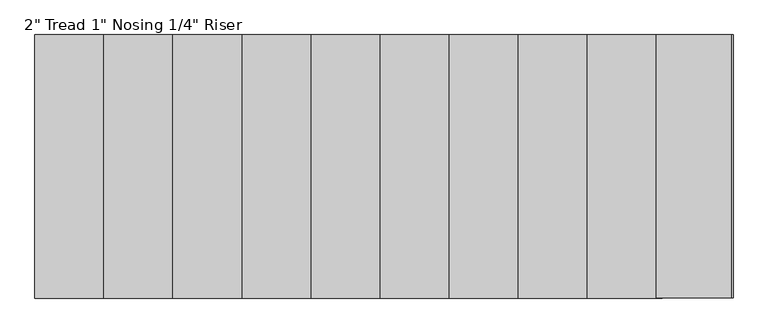
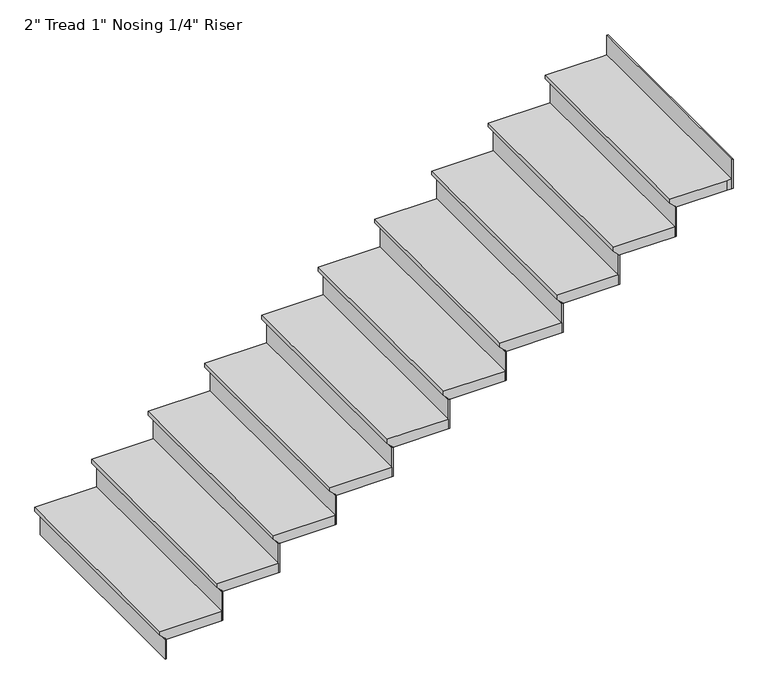
"""IFC4 building model written with IfcOpenShell, lengths in millimetres: stair flight geometry."""

from ifc_helpers import new_model, si_unit, origin, place, context, project, spatial, faceted_brep, source, transform, mapped, element, save


def stair_flight_cc90426c(model_context):
    return source(origin(), model_context, "Body", "Brep", [
        faceted_brep([(-459.26646, -1849.1834702, 133.35), (-459.26646, -1849.1834702, 152.4), (-459.26646, -782.3834702, 152.4), (-459.26646, -782.3834702, 133.35), (-433.86646, -1849.1834702, 107.95), (-433.86646, -782.3834702, 107.95), (-154.46646, -1849.1834702, 152.4), (-154.46646, -782.3834702, 152.4), (-433.86646, -782.3834702, 101.6), (-154.46646, -782.3834702, 101.6), (-154.46646, -1849.1834702, 101.6), (-433.86646, -1849.1834702, 101.6)], [[[0, 1, 2, 3]], [[4, 0, 3, 5]], [[2, 1, 6, 7]], [[8, 9, 10, 11]], [[2, 7, 9, 8, 5, 3]], [[8, 11, 4, 5]], [[6, 1, 0, 4, 11, 10]], [[7, 6, 10, 9]]]),
        faceted_brep([(-433.86646, -1849.1834702, 101.6), (-433.86646, -1849.1834702, 0.0), (-427.51646, -1849.1834702, 0.0), (-427.51646, -1849.1834702, 101.6), (-433.86646, -782.3834702, 101.6), (-427.51646, -782.3834702, 101.6), (-427.51646, -782.3834702, 0.0), (-433.86646, -782.3834702, 0.0)], [[[0, 1, 2, 3]], [[4, 5, 6, 7]], [[1, 0, 4, 7]], [[2, 1, 7, 6]], [[3, 2, 6, 5]], [[0, 3, 5, 4]]]),
        faceted_brep([(-154.46646, -1849.1834702, 254.0), (-154.46646, -1849.1834702, 101.6), (-148.11646, -1849.1834702, 101.6), (-148.11646, -1849.1834702, 254.0), (-154.46646, -782.3834702, 254.0), (-148.11646, -782.3834702, 254.0), (-148.11646, -782.3834702, 101.6), (-154.46646, -782.3834702, 101.6)], [[[0, 1, 2, 3]], [[4, 5, 6, 7]], [[1, 0, 4, 7]], [[2, 1, 7, 6]], [[3, 2, 6, 5]], [[0, 3, 5, 4]]]),
        faceted_brep([(-179.86646, -782.3834702, 304.8), (-179.86646, -1849.1834702, 304.8), (124.93354, -1849.1834702, 304.8), (124.93354, -782.3834702, 304.8), (-154.46646, -782.3834702, 254.0), (124.93354, -782.3834702, 254.0), (124.93354, -1849.1834702, 254.0), (-154.46646, -1849.1834702, 254.0), (-154.46646, -782.3834702, 260.35), (-179.86646, -782.3834702, 285.75), (-154.46646, -1849.1834702, 260.35), (-179.86646, -1849.1834702, 285.75)], [[[0, 1, 2, 3]], [[4, 5, 6, 7]], [[0, 3, 5, 4, 8, 9]], [[4, 7, 10, 8]], [[2, 1, 11, 10, 7, 6]], [[3, 2, 6, 5]], [[11, 1, 0, 9]], [[10, 11, 9, 8]]]),
        faceted_brep([(124.93354, -1849.1834702, 406.4), (124.93354, -1849.1834702, 254.0), (131.28354, -1849.1834702, 254.0), (131.28354, -1849.1834702, 406.4), (124.93354, -782.3834702, 406.4), (131.28354, -782.3834702, 406.4), (131.28354, -782.3834702, 254.0), (124.93354, -782.3834702, 254.0)], [[[0, 1, 2, 3]], [[4, 5, 6, 7]], [[1, 0, 4, 7]], [[2, 1, 7, 6]], [[3, 2, 6, 5]], [[0, 3, 5, 4]]]),
        faceted_brep([(99.53354, -782.3834702, 457.2), (99.53354, -1849.1834702, 457.2), (404.33354, -1849.1834702, 457.2), (404.33354, -782.3834702, 457.2), (124.93354, -782.3834702, 406.4), (404.33354, -782.3834702, 406.4), (404.33354, -1849.1834702, 406.4), (124.93354, -1849.1834702, 406.4), (124.93354, -782.3834702, 412.75), (99.53354, -782.3834702, 438.15), (124.93354, -1849.1834702, 412.75), (99.53354, -1849.1834702, 438.15)], [[[0, 1, 2, 3]], [[4, 5, 6, 7]], [[0, 3, 5, 4, 8, 9]], [[4, 7, 10, 8]], [[2, 1, 11, 10, 7, 6]], [[3, 2, 6, 5]], [[11, 1, 0, 9]], [[10, 11, 9, 8]]]),
        faceted_brep([(404.33354, -1849.1834702, 558.8), (404.33354, -1849.1834702, 406.4), (410.68354, -1849.1834702, 406.4), (410.68354, -1849.1834702, 558.8), (404.33354, -782.3834702, 558.8), (410.68354, -782.3834702, 558.8), (410.68354, -782.3834702, 406.4), (404.33354, -782.3834702, 406.4)], [[[0, 1, 2, 3]], [[4, 5, 6, 7]], [[1, 0, 4, 7]], [[2, 1, 7, 6]], [[3, 2, 6, 5]], [[0, 3, 5, 4]]]),
        faceted_brep([(378.93354, -782.3834702, 609.6), (378.93354, -1849.1834702, 609.6), (683.73354, -1849.1834702, 609.6), (683.73354, -782.3834702, 609.6), (404.33354, -782.3834702, 558.8), (683.73354, -782.3834702, 558.8), (683.73354, -1849.1834702, 558.8), (404.33354, -1849.1834702, 558.8), (404.33354, -782.3834702, 565.15), (378.93354, -782.3834702, 590.55), (404.33354, -1849.1834702, 565.15), (378.93354, -1849.1834702, 590.55)], [[[0, 1, 2, 3]], [[4, 5, 6, 7]], [[0, 3, 5, 4, 8, 9]], [[4, 7, 10, 8]], [[2, 1, 11, 10, 7, 6]], [[3, 2, 6, 5]], [[11, 1, 0, 9]], [[10, 11, 9, 8]]]),
        faceted_brep([(683.73354, -1849.1834702, 711.2), (683.73354, -1849.1834702, 558.8), (690.08354, -1849.1834702, 558.8), (690.08354, -1849.1834702, 711.2), (683.73354, -782.3834702, 711.2), (690.08354, -782.3834702, 711.2), (690.08354, -782.3834702, 558.8), (683.73354, -782.3834702, 558.8)], [[[0, 1, 2, 3]], [[4, 5, 6, 7]], [[1, 0, 4, 7]], [[2, 1, 7, 6]], [[3, 2, 6, 5]], [[0, 3, 5, 4]]]),
        faceted_brep([(658.33354, -782.3834702, 762.0), (658.33354, -1849.1834702, 762.0), (963.13354, -1849.1834702, 762.0), (963.13354, -782.3834702, 762.0), (683.73354, -782.3834702, 711.2), (963.13354, -782.3834702, 711.2), (963.13354, -1849.1834702, 711.2), (683.73354, -1849.1834702, 711.2), (683.73354, -782.3834702, 717.55), (658.33354, -782.3834702, 742.95), (683.73354, -1849.1834702, 717.55), (658.33354, -1849.1834702, 742.95)], [[[0, 1, 2, 3]], [[4, 5, 6, 7]], [[0, 3, 5, 4, 8, 9]], [[4, 7, 10, 8]], [[2, 1, 11, 10, 7, 6]], [[3, 2, 6, 5]], [[11, 1, 0, 9]], [[10, 11, 9, 8]]]),
        faceted_brep([(963.13354, -1849.1834702, 863.6), (963.13354, -1849.1834702, 711.2), (969.48354, -1849.1834702, 711.2), (969.48354, -1849.1834702, 863.6), (963.13354, -782.3834702, 863.6), (969.48354, -782.3834702, 863.6), (969.48354, -782.3834702, 711.2), (963.13354, -782.3834702, 711.2)], [[[0, 1, 2, 3]], [[4, 5, 6, 7]], [[1, 0, 4, 7]], [[2, 1, 7, 6]], [[3, 2, 6, 5]], [[0, 3, 5, 4]]]),
        faceted_brep([(937.73354, -782.3834702, 914.4), (937.73354, -1849.1834702, 914.4), (1242.53354, -1849.1834702, 914.4), (1242.53354, -782.3834702, 914.4), (963.13354, -782.3834702, 863.6), (1242.53354, -782.3834702, 863.6), (1242.53354, -1849.1834702, 863.6), (963.13354, -1849.1834702, 863.6), (963.13354, -782.3834702, 869.95), (937.73354, -782.3834702, 895.35), (963.13354, -1849.1834702, 869.95), (937.73354, -1849.1834702, 895.35)], [[[0, 1, 2, 3]], [[4, 5, 6, 7]], [[0, 3, 5, 4, 8, 9]], [[4, 7, 10, 8]], [[2, 1, 11, 10, 7, 6]], [[3, 2, 6, 5]], [[11, 1, 0, 9]], [[10, 11, 9, 8]]]),
        faceted_brep([(1242.53354, -1849.1834702, 1016.0), (1242.53354, -1849.1834702, 863.6), (1248.88354, -1849.1834702, 863.6), (1248.88354, -1849.1834702, 1016.0), (1242.53354, -782.3834702, 1016.0), (1248.88354, -782.3834702, 1016.0), (1248.88354, -782.3834702, 863.6), (1242.53354, -782.3834702, 863.6)], [[[0, 1, 2, 3]], [[4, 5, 6, 7]], [[1, 0, 4, 7]], [[2, 1, 7, 6]], [[3, 2, 6, 5]], [[0, 3, 5, 4]]]),
        faceted_brep([(1217.13354, -782.3834702, 1066.8), (1217.13354, -1849.1834702, 1066.8), (1521.93354, -1849.1834702, 1066.8), (1521.93354, -782.3834702, 1066.8), (1242.53354, -782.3834702, 1016.0), (1521.93354, -782.3834702, 1016.0), (1521.93354, -1849.1834702, 1016.0), (1242.53354, -1849.1834702, 1016.0), (1242.53354, -782.3834702, 1022.35), (1217.13354, -782.3834702, 1047.75), (1242.53354, -1849.1834702, 1022.35), (1217.13354, -1849.1834702, 1047.75)], [[[0, 1, 2, 3]], [[4, 5, 6, 7]], [[0, 3, 5, 4, 8, 9]], [[4, 7, 10, 8]], [[2, 1, 11, 10, 7, 6]], [[3, 2, 6, 5]], [[11, 1, 0, 9]], [[10, 11, 9, 8]]]),
        faceted_brep([(1521.93354, -1849.1834702, 1168.4), (1521.93354, -1849.1834702, 1016.0), (1528.28354, -1849.1834702, 1016.0), (1528.28354, -1849.1834702, 1168.4), (1521.93354, -782.3834702, 1168.4), (1528.28354, -782.3834702, 1168.4), (1528.28354, -782.3834702, 1016.0), (1521.93354, -782.3834702, 1016.0)], [[[0, 1, 2, 3]], [[4, 5, 6, 7]], [[1, 0, 4, 7]], [[2, 1, 7, 6]], [[3, 2, 6, 5]], [[0, 3, 5, 4]]]),
        faceted_brep([(1496.53354, -782.3834702, 1219.2), (1496.53354, -1849.1834702, 1219.2), (1801.33354, -1849.1834702, 1219.2), (1801.33354, -782.3834702, 1219.2), (1521.93354, -782.3834702, 1168.4), (1801.33354, -782.3834702, 1168.4), (1801.33354, -1849.1834702, 1168.4), (1521.93354, -1849.1834702, 1168.4), (1521.93354, -782.3834702, 1174.75), (1496.53354, -782.3834702, 1200.15), (1521.93354, -1849.1834702, 1174.75), (1496.53354, -1849.1834702, 1200.15)], [[[0, 1, 2, 3]], [[4, 5, 6, 7]], [[0, 3, 5, 4, 8, 9]], [[4, 7, 10, 8]], [[2, 1, 11, 10, 7, 6]], [[3, 2, 6, 5]], [[11, 1, 0, 9]], [[10, 11, 9, 8]]]),
        faceted_brep([(1801.33354, -1849.1834702, 1320.8), (1801.33354, -1849.1834702, 1168.4), (1807.68354, -1849.1834702, 1168.4), (1807.68354, -1849.1834702, 1320.8), (1801.33354, -782.3834702, 1320.8), (1807.68354, -782.3834702, 1320.8), (1807.68354, -782.3834702, 1168.4), (1801.33354, -782.3834702, 1168.4)], [[[0, 1, 2, 3]], [[4, 5, 6, 7]], [[1, 0, 4, 7]], [[2, 1, 7, 6]], [[3, 2, 6, 5]], [[0, 3, 5, 4]]]),
        faceted_brep([(1775.93354, -782.3834702, 1371.6), (1775.93354, -1849.1834702, 1371.6), (2080.73354, -1849.1834702, 1371.6), (2080.73354, -782.3834702, 1371.6), (1801.33354, -782.3834702, 1320.8), (2080.73354, -782.3834702, 1320.8), (2080.73354, -1849.1834702, 1320.8), (1801.33354, -1849.1834702, 1320.8), (1801.33354, -782.3834702, 1327.15), (1775.93354, -782.3834702, 1352.55), (1801.33354, -1849.1834702, 1327.15), (1775.93354, -1849.1834702, 1352.55)], [[[0, 1, 2, 3]], [[4, 5, 6, 7]], [[0, 3, 5, 4, 8, 9]], [[4, 7, 10, 8]], [[2, 1, 11, 10, 7, 6]], [[3, 2, 6, 5]], [[11, 1, 0, 9]], [[10, 11, 9, 8]]]),
        faceted_brep([(2360.13354, -1849.1834702, 1625.6), (2360.13354, -1849.1834702, 1473.2), (2366.48354, -1849.1834702, 1473.2), (2366.48354, -1849.1834702, 1625.6), (2360.13354, -782.3834702, 1625.6), (2366.48354, -782.3834702, 1625.6), (2366.48354, -782.3834702, 1473.2), (2360.13354, -782.3834702, 1473.2)], [[[0, 1, 2, 3]], [[4, 5, 6, 7]], [[1, 0, 4, 7]], [[2, 1, 7, 6]], [[3, 2, 6, 5]], [[0, 3, 5, 4]]]),
        faceted_brep([(2080.73354, -1849.1834702, 1473.2), (2080.73354, -1849.1834702, 1320.8), (2087.08354, -1849.1834702, 1320.8), (2087.08354, -1849.1834702, 1473.2), (2080.73354, -782.3834702, 1473.2), (2087.08354, -782.3834702, 1473.2), (2087.08354, -782.3834702, 1320.8), (2080.73354, -782.3834702, 1320.8)], [[[0, 1, 2, 3]], [[4, 5, 6, 7]], [[1, 0, 4, 7]], [[2, 1, 7, 6]], [[3, 2, 6, 5]], [[0, 3, 5, 4]]]),
        faceted_brep([(2360.13354, -782.3834702, 1524.0), (2334.73354, -782.3834702, 1524.0), (2055.33354, -782.3834702, 1524.0), (2055.33354, -1849.1834702, 1524.0), (2334.73354, -1849.1834702, 1524.0), (2360.13354, -1849.1834702, 1524.0), (2334.73354, -782.3834702, 1473.2), (2360.13354, -782.3834702, 1473.2), (2360.13354, -1849.1834702, 1473.2), (2334.73354, -1849.1834702, 1473.2), (2080.73354, -1849.1834702, 1473.2), (2080.73354, -782.3834702, 1473.2), (2080.73354, -782.3834702, 1479.55), (2055.33354, -782.3834702, 1504.95), (2080.73354, -1849.1834702, 1479.55), (2055.33354, -1849.1834702, 1504.95)], [[[0, 1, 2, 3, 4, 5]], [[6, 7, 8, 9, 10, 11]], [[1, 0, 7, 6]], [[2, 1, 6, 11, 12, 13]], [[11, 10, 14, 12]], [[4, 3, 15, 14, 10, 9]], [[5, 4, 9, 8]], [[0, 5, 8, 7]], [[15, 3, 2, 13]], [[14, 15, 13, 12]]]),
    ])


if __name__ == "__main__":
    model = new_model("IFC4")
    model_context = context("Model", 3, world=origin())
    ifc_project = project(units=[si_unit("LENGTHUNIT", "METRE", prefix="MILLI")], contexts=[model_context])
    site = spatial("IfcSite", under=ifc_project)
    building = spatial("IfcBuilding", under=site)
    placement = place(None, origin())
    stair_flight_shape = stair_flight_cc90426c(model_context)
    element("IfcStairFlight", 1, ObjectType="2\" Tread 1\" Nosing 1/4\" Riser", at=placement, inside=building, context=model_context, shape_type="MappedRepresentation", body=[
        mapped(stair_flight_shape, transform((0.0, 0.0, 0.0), x_axis=(1.0, 0.0, 0.0), y_axis=(0.0, 1.0, 0.0), z_axis=(0.0, 0.0, 1.0))),
    ])
    save(model, "model.ifc")
